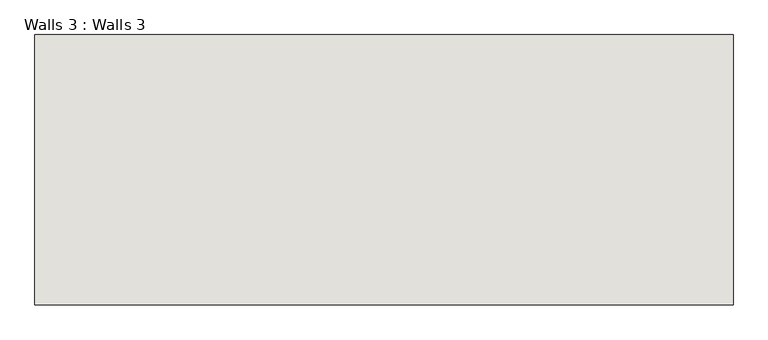
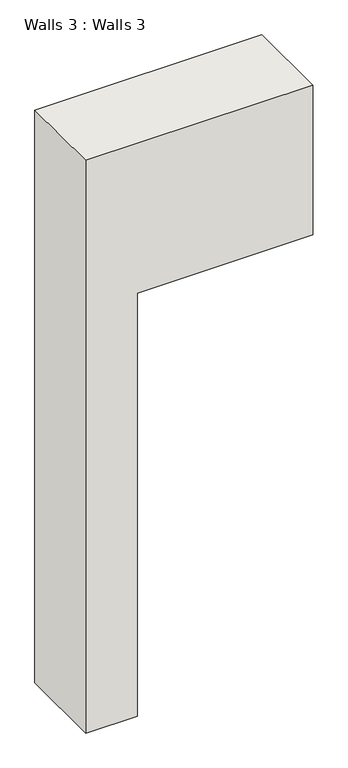
"""IFC4 building model written with IfcOpenShell, lengths in millimetres: wall geometry, Walls 3 : Walls 3."""

from ifc_helpers import new_model, si_unit, frame, origin, place, context, project, spatial, polyline, outline, extrude, source, transform, mapped, element, save


def walls_3_walls_3_66379a57(model_context):
    return source(origin(), model_context, "Body", "SweptSolid", [
        extrude(outline(polyline([(4470.4, -11208.6620963), (0.0, -11208.6620963), (0.0, -10827.6620963), (3302.0, -10827.6620963), (3302.0, -9532.2620963), (4470.4, -9532.2620963), (4470.4, -11208.6620963)])), frame((0.0, -3645.4718653, 0.0), z_axis=(0.0, 1.0, 0.0), x_axis=(0.0, 0.0, 1.0)), (0.0, 0.0, 1.0), 648.7245351),
    ])


if __name__ == "__main__":
    model = new_model("IFC4")
    model_context = context("Model", 3, world=origin())
    ifc_project = project(units=[si_unit("LENGTHUNIT", "METRE", prefix="MILLI")], contexts=[model_context])
    site = spatial("IfcSite", under=ifc_project)
    building = spatial("IfcBuilding", under=site)
    placement = place(None, origin())
    walls_3_walls_3_shape = walls_3_walls_3_66379a57(model_context)
    element("IfcWall", 1, ObjectType="Walls 3 : Walls 3", at=placement, inside=building, context=model_context, shape_type="MappedRepresentation", body=[
        mapped(walls_3_walls_3_shape, transform((0.0, 0.0, 0.0), x_axis=(1.0, 0.0, 0.0), y_axis=(0.0, 1.0, 0.0), z_axis=(0.0, 0.0, 1.0))),
    ])
    save(model, "model.ifc")

# Revit data of these elements
# Element 1 (IfcWall, "Walls 3 : Walls 3")
#   Materials on its faces: "Default Wall"
# Materials
#   "Default Wall": colour RGB 128 128 128, transparency 0
